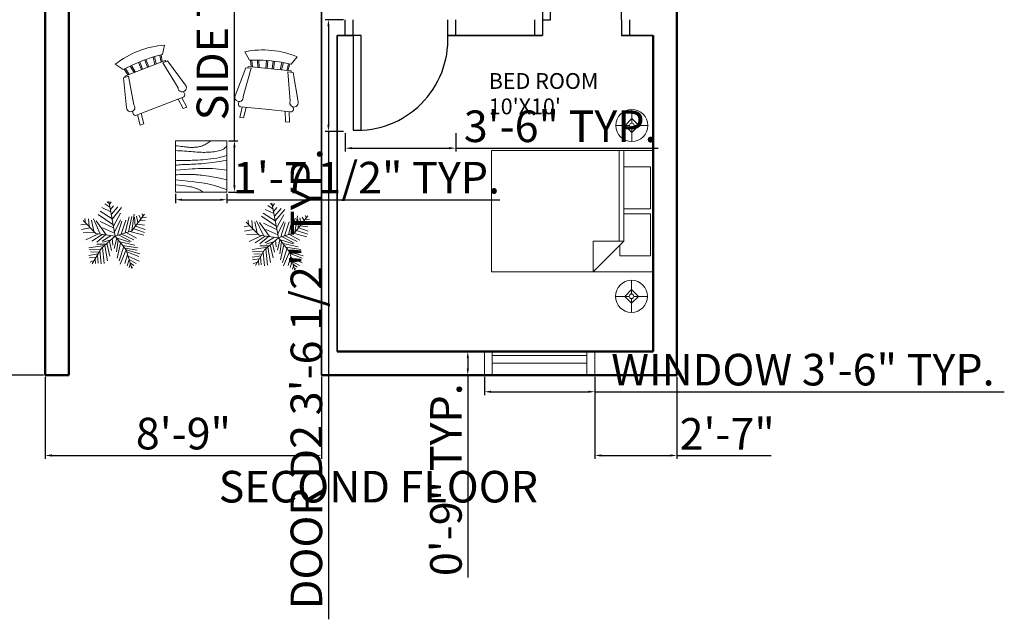
# Model space of a CAD drawing. Units: inches. Extents: x 2296 to 3335, y 495 to 1294.
# Tile 5 of 7: x 2952 to 3326, y 495 to 723. Entities that reach past the tile are written whole.
import ezdxf

# ---------------------------------------------------------------- set-up
doc = ezdxf.new("R2010")
doc.units = ezdxf.units.IN
for name, color, linetype, lineweight in [('A-ANNO-DIMS', 2, 'Continuous', 18), ('A-ANNO-TEXT', 7, 'Continuous', 35), ('A-AREA-IDEN', 7, 'Continuous', 18), ('DOORS', 1, 'Continuous', 25), ('E-LITE', 2, 'Continuous', 18), ('FURNITURE', 2, 'Continuous', 18), ('INNER WALL', 6, 'Continuous', 35), ('L-PLNT', 3, 'Continuous', 13), ('OUTER WALL', 5, 'Continuous', 50), ('WINDOWS', 3, 'Continuous', 18)]:
    doc.layers.add(name, color=color, linetype=linetype, lineweight=lineweight)
doc.styles.get("Standard").update_dxf_attribs({"font": 'arial.ttf'})
doc.dimstyles.new('ISO-25', dxfattribs={"dimtxt": 12, "dimasz": 2.5, "dimexe": 1.25, "dimexo": 0.625, "dimtad": 1, "dimdec": 1, "dimlunit": 3, "dimtxsty": 'Standard', "dimcen": 2.5, "dimadec": 0, "dimazin": 0, "dimtfac": 1, "dimtdec": 1, "dimtmove": 0, "dimatfit": 3, "dimfxl": 1, "dimarcsym": 0})

# ---------------------------------------------------------------- blocks, each defined once
blk = doc.blocks.new('Chair - Rocking')
for p, q in [((-8, -4.5), (-10, -1.5)), ((8, -4.5), (10, -1.5)), ((-8.23428, -6.99939), (-8.3093, -7.47958)), ((-8.23041, -7), (8.23915, -7)), ((-7.5, -4.5), (-7, -7)), ((-6.5, -7), (-7.02225, -4.43)), ((-4.5, -7), (-4.96674, -4.19951)), ((-4, -7), (-4.40532, -4.16272)), ((-1.5, -4.05012), (-1.5, -7)), ((-1, -7), (-1, -4.05012)), ((1, -7), (1, -4.04655)), ((1.5, -4.05012), (1.5, -7)), ((4, -7), (4.40187, -4.18694)), ((4.5, -7), (4.96761, -4.19437)), ((6.5, -7), (7, -4.4057)), ((7.5, -4.5), (7, -7)), ((8.31071, -7.48854), (8.23449, -7.00073)), ((-9, -7.5), (-12, -18.49999)), ((-7, -7.5), (-9, -7.5)), ((-9, -18.49999), (-7, -7.5)), ((7, -7.5), (9, -7.5)), ((9, -18.49999), (7, -7.5)), ((9, -7.5), (12, -18.49999)), ((-10.36644, -20.64523), (-10.5, -21.49999)), ((10.5, -21.49999), (10.3575, -20.58798)), ((-9, -22.49999), (-9.5, -26.49999)), ((0, -22.49999), (-9.5, -22.49999)), ((-8, -26.49999), (-7.5, -22.49999)), ((0, -22.49999), (9.5, -22.49999)), ((8, -26.49999), (7.5, -22.49999)), ((9, -22.49999), (9.5, -26.49999)), ((-9.5, -26.49999), (-8, -26.49999)), ((9.5, -26.49999), (8, -26.49999))]:
    blk.add_line(p, q)
for centre, radius, start, end in [((0, -34.08333), 34.08333, 72.93847, 107.0615), ((0, -68.25004), 64.25, 93.92211, 97.15267), ((0, -68.25004), 64.25, 82.84733, 93.92211), ((-10.5, -18.99999), 1.58114, 161.5651, 18.43495), ((10.5, -18.99999), 1.58114, 161.5651, 18.43495), ((-9.5, -21.49999), 1, 180, 270), ((9.5, -21.49999), 1, 270, 0)]:
    blk.add_arc(centre, radius, start, end)
blk = doc.blocks.new('Table - Square Woodgrain 42 x 42 in.')
blk.add_line((0, -42), (42, -42))
for points in [[(0, -4), (1.704, -4.2172), (3.2358, -4.4188), (4.615, -4.604), (5.8615, -4.7721), (6.9951, -4.9224), (8.0357, -5.0541), (9.0031, -5.1667), (9.9171, -5.2594), (10.7951, -5.3316), (11.6445, -5.3836), (12.4702, -5.4157), (13.277, -5.4283), (14.0698, -5.4217), (14.8535, -5.3964), (15.6331, -5.3526), (16.4133, -5.2908), (17.1986, -5.2103), (17.9913, -5.1062), (18.793, -4.9727), (19.6056, -4.8038), (20.4307, -4.5937), (21.2701, -4.3365), (22.1256, -4.0262), (22.9989, -3.6571), (23.888, -3.2272), (24.7756, -2.7516), (25.6408, -2.2491), (26.4624, -1.7387), (27.2195, -1.2395), (27.891, -0.7703), (28.456, -0.3501), (28.8934, 0.002)], [(0, -42), (0, 0), (42, 0), (42, -42)], [(0, -8), (1.8203, -8.1001), (3.6741, -8.2149), (5.5411, -8.3408), (7.4011, -8.4741), (9.2339, -8.6112), (11.0193, -8.7484), (12.7371, -8.8821), (14.3671, -9.0086), (15.8954, -9.1246), (17.3337, -9.2278), (18.6997, -9.3159), (20.0116, -9.387), (21.2871, -9.4389), (22.5442, -9.4696), (23.8008, -9.477), (25.0749, -9.459), (26.3791, -9.4137), (27.7049, -9.3403), (29.0383, -9.2382), (30.3655, -9.1068), (31.6728, -8.9455), (32.9461, -8.7535), (34.1717, -8.5304), (35.3358, -8.2756), (36.4268, -7.9863), (37.443, -7.6521), (38.3849, -7.2603), (39.253, -6.7986), (40.048, -6.2542), (40.7705, -5.6147), (41.421, -4.8674), (42, -4)], [(42, -12), (39.1784, -12.8621), (36.4519, -13.5654), (33.8246, -14.1294), (31.3004, -14.5731), (28.8832, -14.9161), (26.577, -15.1775), (24.3858, -15.3768), (22.3136, -15.5332), (20.3622, -15.6632), (18.5254, -15.7718), (16.7947, -15.8612), (15.1618, -15.9338), (13.6183, -15.9916), (12.1558, -16.0369), (10.7659, -16.0718), (9.4403, -16.0987), (8.1703, -16.1191), (6.9461, -16.1325), (5.7577, -16.1377), (4.595, -16.1335), (3.4479, -16.1188), (2.3064, -16.0924), (1.1604, -16.0532), (0, -16)], [(42, -16), (37.6529, -16.7365), (33.8802, -17.329), (30.6179, -17.7961), (27.8015, -18.1561), (25.3668, -18.4275), (23.2497, -18.6288), (21.3859, -18.7785), (19.7111, -18.8949), (18.1693, -18.9939), (16.7375, -19.0795), (15.401, -19.1534), (14.1449, -19.217), (12.9544, -19.2717), (11.8148, -19.3191), (10.7113, -19.3606), (9.6291, -19.3976), (8.5534, -19.4323), (7.47, -19.4689), (6.3643, -19.5122), (5.222, -19.5672), (4.0288, -19.6386), (2.7703, -19.7313), (1.4321, -19.8501), (0, -20)], [(0, -24), (3.9243, -23.6805), (7.4766, -23.4138), (10.6891, -23.1954), (13.5943, -23.0205), (16.2247, -22.8847), (18.6125, -22.7832), (20.7903, -22.7116), (22.7903, -22.6651), (24.6563, -22.642), (26.4764, -22.6507), (28.35, -22.7024), (30.3766, -22.8084), (32.6555, -22.98), (35.2861, -23.2283), (38.3678, -23.5645), (42, -24)], [(42, -32), (37.392, -31.017), (33.4585, -30.2231), (30.1291, -29.5949), (27.3334, -29.109), (25.0009, -28.742), (23.0612, -28.4707), (21.4439, -28.2716), (20.0786, -28.1215), (18.8998, -28.0002), (17.8609, -27.9014), (16.9206, -27.8219), (16.0371, -27.7588), (15.1691, -27.709), (14.2748, -27.6693), (13.3128, -27.6368), (12.2415, -27.6083), (11.0295, -27.5824), (9.6867, -27.5643), (8.233, -27.5608), (6.6884, -27.5787), (5.0728, -27.6248), (3.4062, -27.7058), (1.7086, -27.8286), (0, -28)], [(0, -32), (5.4026, -32.5358), (9.9494, -33.019), (13.7424, -33.4553), (16.8834, -33.8505), (19.4743, -34.2106), (21.6171, -34.5413), (23.4136, -34.8486), (24.9657, -35.1382), (26.3614, -35.4156), (27.6332, -35.6841), (28.7995, -35.9467), (29.8788, -36.2064), (30.8897, -36.4661), (31.8507, -36.7288), (32.7802, -36.9973), (33.6968, -37.2747), (34.6175, -37.5635), (35.5531, -37.8651), (36.5128, -38.1805), (37.506, -38.5108), (38.5421, -38.8568), (39.6302, -39.2197), (40.7797, -39.6004), (42, -40)], [(0, -36), (3.0098, -36.2857), (5.5354, -36.5643), (7.6368, -36.8359), (9.374, -37.1009), (10.807, -37.3597), (11.9957, -37.6126), (13.0002, -37.8599), (13.8804, -38.102), (14.6874, -38.3393), (15.4365, -38.5729), (16.1338, -38.8041), (16.7858, -39.0341), (17.3987, -39.264), (17.9787, -39.4952), (18.5322, -39.7288), (19.0655, -39.9662), (19.5832, -40.2081), (20.0842, -40.4544), (20.5657, -40.7046), (21.0249, -40.9581), (21.459, -41.2144), (21.8653, -41.4731), (22.2409, -41.7335), (22.5831, -41.9951)]]:
    blk.add_lwpolyline(points)
blk = doc.blocks.new('Bed - Queen')
for p, q in [((0, -80.00003), (0, 0)), ((0, 0), (59.99999, 0)), ((59.99999, 0), (59.99999, -80.00003)), ((7.99999, -1.2), (28.79998, -1.2)), ((7.99999, -14.4), (7.99999, -1.2)), ((28.79998, -1.2), (28.79998, -14.4)), ((31.19999, -1.2), (51.99999, -1.2)), ((31.19999, -14.4), (31.19999, -1.2)), ((51.99999, -1.2), (51.99999, -16.4)), ((0, -14.4), (44.8, -14.4)), ((59.99999, -29.6), (44.8, -14.4)), ((44.8, -14.4), (44.8, -29.6)), ((44.8, -16.8), (0, -16.8)), ((51.99999, -16.4), (46.79936, -16.4)), ((44.8, -29.6), (59.99999, -29.6)), ((59.99999, -80.00003), (0, -80.00003))]:
    blk.add_line(p, q)
blk = doc.blocks.new('Lamp - Table')
for p, q in [((0, 7), (0, 1)), ((-1, 0), (-7, 0)), ((0, 3), (-3, 0)), ((-3, 0), (0, -3)), ((3, 0), (0, 3)), ((0, -3), (3, 0)), ((1, 0), (7, 0)), ((0, -1), (0, -7))]:
    blk.add_line(p, q)
for radius in [7, 1]:
    blk.add_circle((0, 0), radius)
blk = doc.blocks.new('*U15')
for p, q in [((-8.737, 47.138), (-17.069, 52.711)), ((-10.186, 53.64), (-13.084, 55.962)), ((0, 0), (-10.5, 57)), ((-9.099, 51.782), (-6.563, 55.962)), ((-7.65, 43.423), (-2.578, 49.46)), ((-3.665, 19.273), (-27.574, 35.527)), ((-5.114, 28.097), (-24.676, 40.636)), ((-7.288, 39.707), (-21.778, 46.673)), ((-5.839, 35.992), (4.667, 48.067)), ((-5.114, 27.632), (10.463, 46.673)), ((-2.941, 16.486), (8.652, 37.85)), ((22.055, 7.198), (27.489, 32.277)), ((27, 9), (48, 36)), ((27.127, 9.056), (31.112, 35.992)), ((35.096, 32.741), (37.27, 22.524)), ((38.719, 34.134), (41.979, 28.561)), ((44.153, 36.456), (45.239, 32.741)), ((-47.498, 19.737), (-55.83, 18.344)), ((-31.5, 4.5), (-52.5, 25.5)), ((-48.585, 21.131), (-49.309, 29.026)), ((-43.513, 28.561), (-42.427, 15.558)), ((-38.442, 26.239), (-34.819, 7.663)), ((-35.544, 28.097), (-24.314, 3.947)), ((-14.533, 2.09), (-30.834, 25.31)), ((-24.314, 23.917), (-2.941, 13.7)), ((-1.129, 6.734), (9.014, 26.704)), ((3.942, 1.625), (11.187, 24.381)), ((10.101, 3.483), (17.708, 26.239)), ((16.259, 5.805), (23.142, 31.348)), ((31.836, 30.883), (32.561, 16.486)), ((33.285, 16.486), (48.862, 10.913)), ((36.183, 19.737), (48.137, 17.88)), ((40.53, 25.775), (48.862, 24.846)), ((43.791, 29.954), (51.036, 30.883)), ((-40.615, 13.7), (-55.105, 10.913)), ((-33.37, 6.269), (-52.207, 5.34)), ((-28.299, 3.483), (-47.86, -5.805)), ((-21.416, 3.018), (-38.079, -8.128)), ((0, 0), (-31.5, 4.5)), ((-15.982, 2.09), (-30.11, -9.521)), ((0, 0), (-22.5, -19.5)), ((-6.563, 1.161), (-21.416, -8.128)), ((-20.691, 13.7), (-1.129, 4.876)), ((0, 0), (27, 9)), ((0, 0), (18, -22.5)), ((6.478, 1.625), (26.04, -8.592)), ((11.187, 3.483), (30.749, -5.805)), ((18.07, 5.805), (35.096, -3.483)), ((24.229, 7.663), (46.688, 1.625)), ((29.662, 12.307), (48.137, 6.269)), ((-17.431, -15.094), (-42.789, -18.809)), ((-15.257, -12.772), (-30.11, -12.772)), ((-6.563, -5.805), (-19.967, -9.985)), ((-17.069, -15.094), (-12.721, -40.172)), ((-13.446, -11.378), (-8.737, -32.741)), ((-9.461, -8.592), (-6.201, -23.453)), ((-4.752, -3.483), (-3.665, -14.629)), ((2.493, -3.019), (-1.491, -20.202)), ((1.769, -2.555), (24.229, -9.521)), ((5.029, -6.27), (2.131, -25.775)), ((9.014, -11.378), (3.58, -35.992)), ((7.565, -9.056), (32.198, -14.629)), ((12.274, -15.094), (36.907, -18.809)), ((-28.299, -29.026), (-42.789, -31.348)), ((-24.314, -21.596), (-42.427, -22.06)), ((-26.849, -26.24), (-40.253, -25.775)), ((-22.5, -19.5), (-37.5, -45)), ((-29.023, -30.884), (-27.936, -43.887)), ((-25.038, -23.918), (-22.865, -45.281)), ((-20.691, -18.345), (-17.793, -44.352)), ((14.085, -16.951), (6.478, -40.172)), ((18.07, -22.524), (8.289, -45.745)), ((20.244, -30.419), (15.897, -44.816)), ((16.259, -19.738), (36.183, -22.989)), ((18, -22.5), (27, -52.5)), ((18.433, -22.524), (40.53, -29.026)), ((19.157, -25.311), (38.719, -33.206)), ((-30.834, -34.135), (-42.427, -35.528)), ((-34.457, -39.708), (-40.978, -42.494)), ((-32.646, -36.921), (-31.921, -44.352)), ((22.78, -37.85), (19.519, -48.532)), ((21.331, -32.741), (39.081, -40.636)), ((22.78, -38.314), (34.372, -44.816)), ((24.591, -45.745), (23.142, -50.854)), ((24.591, -43.423), (30.749, -47.603)), ((26.764, -49.925), (28.213, -50.854))]:
    blk.add_line(p, q)
blk = doc.blocks.new('DOOR-SINGLE-30IN')
for p, q in [((-3, 0), (-3, -6)), ((0, 0), (0, -6)), ((30, 0), (30, -6)), ((33, 0), (33, -6))]:
    blk.add_line(p, q)
blk.add_lwpolyline([(0, 0), (3, 0), (3, 30), (0, 30)], close=True)
blk.add_arc((1.5, 1.5), 28.54, 356.9872, 93.0128)
blk = doc.blocks.new('DOOR-SINGLE-36IN')
for p, q in [((0, 39), (-6, 39)), ((0, 36), (-6, 36)), ((0, 0), (-6, 0)), ((0, -3), (-6, -3))]:
    blk.add_line(p, q)
blk.add_lwpolyline([(0, 0), (36, 0), (36, 3), (0, 3)], close=True)
blk.add_arc((1.5, 1.5), 34.53, 357.5104, 92.4896)
blk = doc.blocks.new('WIN-36IN')
for p, q in [((0, 42), (9, 42)), ((0, 39), (9, 39)), ((1.5, 3), (1.5, 39)), ((4.5, 3), (4.5, 39)), ((9, 3), (0, 3)), ((9, 0), (0, 0))]:
    blk.add_line(p, q)
blk = doc.blocks.new('*D35')
at = {"layer": 'A-ANNO-DIMS', "color": 0, "lineweight": -2, "transparency": 16777216}
for p, q in [((3128.54, 587.39), (3128.54, 580.47)), ((3170.54, 587.39), (3170.54, 580.47)), ((3131.04, 581.72), (3168.04, 581.72)), ((3170.54, 581.72), (3326.14, 581.72))]:
    blk.add_line(p, q, dxfattribs=at)
at = {"layer": 'A-ANNO-DIMS', "color": 0, "transparency": 16777216}
for points in [[(3131.04, 582.13), (3131.04, 581.3), (3128.54, 581.72)], [(3168.04, 582.13), (3168.04, 581.3), (3170.54, 581.72)]]:
    blk.add_solid(points, dxfattribs=at)
at = {"layer": 'Defpoints', "color": 0, "transparency": 16777216}
for p in [(3128.54, 588.02), (3170.54, 588.02), (3170.54, 581.72)]:
    blk.add_point(p, dxfattribs=at)
at = {"layer": 'A-ANNO-DIMS', "color": 0, "transparency": 16777216, "insert": (3249.59, 588.56), "char_height": 12, "attachment_point": 5}
blk.add_mtext('WINDOW 3\'-6" TYP.', dxfattribs=at)
blk = doc.blocks.new('*D36')
at = {"layer": 'A-ANNO-DIMS', "color": 0, "lineweight": -2, "transparency": 16777216}
for p, q in [((3127.92, 597.02), (3120.99, 597.02)), ((3122.24, 594.52), (3122.24, 590.52)), ((3127.92, 588.02), (3120.99, 588.02)), ((3122.24, 588.02), (3122.24, 511.12))]:
    blk.add_line(p, q, dxfattribs=at)
at = {"layer": 'A-ANNO-DIMS', "color": 0, "transparency": 16777216}
for points in [[(3121.82, 594.52), (3122.66, 594.52), (3122.24, 597.02)], [(3121.82, 590.52), (3122.66, 590.52), (3122.24, 588.02)]]:
    blk.add_solid(points, dxfattribs=at)
at = {"layer": 'Defpoints', "color": 0, "transparency": 16777216}
for p in [(3128.54, 597.02), (3122.24, 588.02), (3128.54, 588.02)]:
    blk.add_point(p, dxfattribs=at)
at = {"layer": 'A-ANNO-DIMS', "color": 0, "transparency": 16777216, "insert": (3115.49, 548.32), "char_height": 12, "attachment_point": 5, "rotation": 90}
blk.add_mtext('0\'-9" TYP.', dxfattribs=at)
blk = doc.blocks.new('*D39')
at = {"layer": 'A-ANNO-DIMS', "color": 0, "lineweight": -2, "transparency": 16777216}
for p, q in [((3075.02, 723.02), (3068.03, 723.02)), ((3069.28, 720.52), (3069.28, 683.1)), ((3075.02, 680.6), (3068.03, 680.6)), ((3069.28, 680.6), (3069.28, 495.3))]:
    blk.add_line(p, q, dxfattribs=at)
at = {"layer": 'A-ANNO-DIMS', "color": 0, "transparency": 16777216}
for points in [[(3068.87, 720.52), (3069.7, 720.52), (3069.28, 723.02)], [(3068.87, 683.1), (3069.7, 683.1), (3069.28, 680.6)]]:
    blk.add_solid(points, dxfattribs=at)
at = {"layer": 'Defpoints', "color": 0, "transparency": 16777216}
for p in [(3075.65, 723.02), (3069.28, 680.6), (3075.65, 680.6)]:
    blk.add_point(p, dxfattribs=at)
at = {"layer": 'A-ANNO-DIMS', "color": 0, "transparency": 16777216, "insert": (3062.45, 586.7), "char_height": 12, "attachment_point": 5, "rotation": 90}
blk.add_mtext('DOOR D2 3\'-6 1/2" TYP.', dxfattribs=at)
blk = doc.blocks.new('*D40')
at = {"layer": 'A-ANNO-DIMS', "color": 0, "lineweight": -2, "transparency": 16777216}
for p, q in [((3075.65, 679.97), (3075.65, 672.98)), ((3117.65, 679.97), (3117.65, 672.98)), ((3078.15, 674.23), (3115.15, 674.23)), ((3117.65, 674.23), (3194.53, 674.23))]:
    blk.add_line(p, q, dxfattribs=at)
at = {"layer": 'A-ANNO-DIMS', "color": 0, "transparency": 16777216}
for points in [[(3078.15, 674.65), (3078.15, 673.82), (3075.65, 674.23)], [(3115.15, 674.65), (3115.15, 673.82), (3117.65, 674.23)]]:
    blk.add_solid(points, dxfattribs=at)
at = {"layer": 'Defpoints', "color": 0, "transparency": 16777216}
for p in [(3075.65, 680.6), (3117.65, 680.6), (3117.65, 674.23)]:
    blk.add_point(p, dxfattribs=at)
at = {"layer": 'A-ANNO-DIMS', "color": 0, "transparency": 16777216, "insert": (3157.34, 680.99), "char_height": 12, "attachment_point": 5}
blk.add_mtext('3\'-6" TYP.', dxfattribs=at)
blk = doc.blocks.new('*D49')
at = {"layer": 'A-ANNO-DIMS', "color": 0, "lineweight": -2, "transparency": 16777216}
for p, q in [((3033.55, 677.03), (3033.55, 883.38)), ((3031.26, 677.03), (3034.8, 677.03)), ((3033.55, 660.07), (3033.55, 674.53)), ((3031.26, 657.57), (3034.8, 657.57))]:
    blk.add_line(p, q, dxfattribs=at)
at = {"layer": 'A-ANNO-DIMS', "color": 0, "transparency": 16777216}
for points in [[(3033.13, 674.53), (3033.97, 674.53), (3033.55, 677.03)], [(3033.13, 660.07), (3033.97, 660.07), (3033.55, 657.57)]]:
    blk.add_solid(points, dxfattribs=at)
at = {"layer": 'Defpoints', "color": 0, "transparency": 16777216}
for p in [(3030.63, 677.03), (3033.55, 677.03), (3030.63, 657.57)]:
    blk.add_point(p, dxfattribs=at)
at = {"layer": 'A-ANNO-DIMS', "color": 0, "transparency": 16777216, "insert": (3026.72, 781.45), "char_height": 12, "attachment_point": 5, "rotation": 90}
blk.add_mtext('SIDE TABLE 1\'-7 1/2" TYP.', dxfattribs=at)
blk = doc.blocks.new('*D50')
at = {"layer": 'A-ANNO-DIMS', "color": 0, "lineweight": -2, "transparency": 16777216}
for p, q in [((3011.17, 656.94), (3011.17, 653.4)), ((3030.63, 656.94), (3030.63, 653.4)), ((3013.67, 654.65), (3028.13, 654.65)), ((3030.63, 654.65), (3134.36, 654.65))]:
    blk.add_line(p, q, dxfattribs=at)
at = {"layer": 'A-ANNO-DIMS', "color": 0, "transparency": 16777216}
for points in [[(3013.67, 655.07), (3013.67, 654.23), (3011.17, 654.65)], [(3028.13, 655.07), (3028.13, 654.23), (3030.63, 654.65)]]:
    blk.add_solid(points, dxfattribs=at)
at = {"layer": 'Defpoints', "color": 0, "transparency": 16777216}
for p in [(3011.17, 657.57), (3030.63, 657.57), (3030.63, 654.65)]:
    blk.add_point(p, dxfattribs=at)
at = {"layer": 'A-ANNO-DIMS', "color": 0, "transparency": 16777216, "insert": (3083.74, 661.48), "char_height": 12, "attachment_point": 5}
blk.add_mtext('1\'-7 1/2" TYP.', dxfattribs=at)
blk = doc.blocks.new('*D54')
at = {"layer": 'A-ANNO-DIMS', "color": 0, "lineweight": -2, "transparency": 16777216}
for p, q in [((2961.02, 1068.02), (2929.9, 1068.02)), ((2931.15, 590.52), (2931.15, 1065.52)), ((2961.02, 588.02), (2929.9, 588.02))]:
    blk.add_line(p, q, dxfattribs=at)
at = {"layer": 'A-ANNO-DIMS', "color": 0, "transparency": 16777216}
for points in [[(2930.73, 1065.52), (2931.56, 1065.52), (2931.15, 1068.02)], [(2930.73, 590.52), (2931.56, 590.52), (2931.15, 588.02)]]:
    blk.add_solid(points, dxfattribs=at)
at = {"layer": 'Defpoints', "color": 0, "transparency": 16777216}
for p in [(2931.15, 1068.02), (2961.65, 1068.02), (2961.65, 588.02)]:
    blk.add_point(p, dxfattribs=at)
at = {"layer": 'A-ANNO-DIMS', "color": 0, "transparency": 16777216, "insert": (2924.39, 828.02), "char_height": 12, "attachment_point": 5, "rotation": 90}
blk.add_mtext('40\'-0"', dxfattribs=at)
blk = doc.blocks.new('*D77')
at = {"layer": 'A-ANNO-DIMS', "color": 0, "lineweight": -2, "transparency": 16777216}
for p, q in [((3170.54, 587.39), (3170.54, 556.27)), ((3201.65, 587.39), (3201.65, 556.27)), ((3173.04, 557.52), (3199.15, 557.52)), ((3201.65, 557.52), (3237.5, 557.52))]:
    blk.add_line(p, q, dxfattribs=at)
at = {"layer": 'A-ANNO-DIMS', "color": 0, "transparency": 16777216}
for points in [[(3173.04, 557.93), (3173.04, 557.1), (3170.54, 557.52)], [(3199.15, 557.93), (3199.15, 557.1), (3201.65, 557.52)]]:
    blk.add_solid(points, dxfattribs=at)
at = {"layer": 'Defpoints', "color": 0, "transparency": 16777216}
for p in [(3170.54, 588.02), (3201.65, 588.02), (3201.65, 557.52)]:
    blk.add_point(p, dxfattribs=at)
at = {"layer": 'A-ANNO-DIMS', "color": 0, "transparency": 16777216, "insert": (3220.82, 564.17), "char_height": 12, "attachment_point": 5}
blk.add_mtext('2\'-7"', dxfattribs=at)
blk = doc.blocks.new('*D78')
at = {"layer": 'A-ANNO-DIMS', "color": 0, "lineweight": -2, "transparency": 16777216}
for p, q in [((2961.65, 587.39), (2961.65, 556.27)), ((3066.65, 587.39), (3066.65, 556.27)), ((2964.15, 557.52), (3064.15, 557.52))]:
    blk.add_line(p, q, dxfattribs=at)
at = {"layer": 'A-ANNO-DIMS', "color": 0, "transparency": 16777216}
for points in [[(2964.15, 557.93), (2964.15, 557.1), (2961.65, 557.52)], [(3064.15, 557.93), (3064.15, 557.1), (3066.65, 557.52)]]:
    blk.add_solid(points, dxfattribs=at)
at = {"layer": 'Defpoints', "color": 0, "transparency": 16777216}
for p in [(2961.65, 588.02), (3066.65, 588.02), (3066.65, 557.52)]:
    blk.add_point(p, dxfattribs=at)
at = {"layer": 'A-ANNO-DIMS', "color": 0, "transparency": 16777216, "insert": (3014.15, 564.27), "char_height": 12, "attachment_point": 5}
blk.add_mtext('8\'-9"', dxfattribs=at)

msp = doc.modelspace()

# ---------------------------------------------------------------- linework, layer by layer
at = {"layer": 'INNER WALL'}
for p, q in [((3066.65, 588.02), (3066.65, 777.02)), ((3072.65, 717.02), (3078.65, 717.02)), ((3072.65, 597.02), (3072.65, 717.02)), ((3114.65, 717.02), (3150.65, 717.02)), ((3180.65, 717.02), (3192.65, 717.02))]:
    msp.add_line(p, q, dxfattribs=at)
at = {"layer": 'OUTER WALL'}
for p, q in [((2970.65, 861.02), (2970.65, 588.02)), ((3192.65, 597.02), (3192.65, 717.02)), ((3072.65, 597.02), (3192.65, 597.02))]:
    msp.add_line(p, q, dxfattribs=at)
msp.add_lwpolyline([(3066.65, 588.02), (3201.65, 588.02), (3201.65, 1068.02), (2961.65, 1068.02), (2961.65, 588.02), (2970.65, 588.02)], dxfattribs=at)

# ---------------------------------------------------------------- block references
at = {"layer": 'DOORS'}
msp.add_blockref('DOOR-SINGLE-30IN', (3150.65, 723.02), dxfattribs=at)
at = {"layer": 'DOORS', "rotation": 269.9999999999998}
msp.add_blockref('DOOR-SINGLE-36IN', (3078.65, 717.02), dxfattribs=at)
at = {"layer": 'E-LITE', "xscale": 0.8700180084150424, "yscale": 0.8700180084150424, "zscale": 0.8700180084150424}
for p in [(3184.6, 682.84), (3184.47, 617.95)]:
    msp.add_blockref('Lamp - Table', p, dxfattribs=at)
at = {"layer": 'FURNITURE'}
for p, rotation in [((2997.07, 711.13), 21.07995296200778), ((3047.62, 711.37), 354.3621064589386)]:
    msp.add_blockref('Chair - Rocking', p, dxfattribs=dict(at, rotation=rotation))
at = {"layer": 'FURNITURE', "xscale": 0.4632804466850307, "yscale": 0.4632804466850307, "zscale": 0.4632804466850307}
msp.add_blockref('Table - Square Woodgrain 42 x 42 in.', (3011.17, 677.03), dxfattribs=at)
at = {"layer": 'FURNITURE', "xscale": 0.7674836837443932, "yscale": 0.7674836837443932, "zscale": 0.7674836837443932, "rotation": 270}
msp.add_blockref('Bed - Queen', (3192.65, 673.29), dxfattribs=at)
at = {"layer": 'L-PLNT', "xscale": 0.232668267563004, "yscale": 0.232668267563004, "zscale": 0.232668267563004}
for p in [(2988.21, 640.8), (3050.25, 640.14)]:
    msp.add_blockref('*U15', p, dxfattribs=at)
at = {"layer": 'WINDOWS', "rotation": 269.9999999999988}
msp.add_blockref('WIN-36IN', (3128.54, 597.02), dxfattribs=at)

# ---------------------------------------------------------------- texts
at = {"layer": 'A-ANNO-TEXT'}
msp.add_text('SECOND FLOOR', height=12, dxfattribs=at).set_placement((3027.56, 539.66))
at = {"layer": 'A-AREA-IDEN'}
for s, p in [('BED ROOM', (3130.2, 696.74)), ("10'X10'", (3130.2, 687.1))]:
    msp.add_text(s, height=6, dxfattribs=at).set_placement(p)

# ---------------------------------------------------------------- dimensions: what is measured, and where the dimension line sits
at = {"layer": 'A-ANNO-DIMS'}
dim = msp.add_linear_dim(base=(2931.15, 1068.02), p1=(2961.65, 588.02), p2=(2961.65, 1068.02), angle=90, dimstyle='ISO-25', override={"dimdec": 1, "dimlfac": 1, "dimrnd": 0, "dimzin": 1, "dimdsep": 46, "dimlunit": 4, "dimfrac": 2}, dxfattribs=at)
dim.commit()
dim.dimension.update_dxf_attribs({"geometry": '*D54', "text_midpoint": (2924.39, 828.02)})
for base, p1, p2, angle, text, picture, middle in [((3033.55, 677.03), (3030.63, 657.57), (3030.63, 677.03), 90, 'SIDE TABLE <> TYP.', '*D49', (3026.72, 781.45)), ((3069.28, 680.6), (3075.65, 723.02), (3075.65, 680.6), 270, 'DOOR D2 <> TYP.', '*D39', (3062.45, 586.7)), ((3122.24, 588.02), (3128.54, 597.02), (3128.54, 588.02), 270, '<> TYP.', '*D36', (3115.49, 548.32))]:
    dim = msp.add_linear_dim(base=base, p1=p1, p2=p2, angle=angle, text=text, dimstyle='ISO-25', override={"dimdec": 1, "dimlfac": 1, "dimrnd": 0, "dimzin": 1, "dimdsep": 46, "dimlunit": 4, "dimfrac": 2}, dxfattribs=at)
    dim.commit()
    dim.dimension.update_dxf_attribs({"geometry": picture, "text_midpoint": middle})
for base, p1, p2, text, picture, middle in [((3117.65, 674.23), (3075.65, 680.6), (3117.65, 680.6), '<> TYP.', '*D40', (3157.34, 680.99)), ((3030.63, 654.65), (3011.17, 657.57), (3030.63, 657.57), '<> TYP.', '*D50', (3083.74, 661.48)), ((3170.54, 581.72), (3128.54, 588.02), (3170.54, 588.02), 'WINDOW <> TYP.', '*D35', (3249.59, 588.56))]:
    dim = msp.add_linear_dim(base=base, p1=p1, p2=p2, text=text, dimstyle='ISO-25', override={"dimdec": 1, "dimlfac": 1, "dimrnd": 0, "dimzin": 1, "dimdsep": 46, "dimlunit": 4, "dimfrac": 2}, dxfattribs=at)
    dim.commit()
    dim.dimension.update_dxf_attribs({"geometry": picture, "text_midpoint": middle})
for base, p1, p2, picture, middle in [((3066.65, 557.52), (2961.65, 588.02), (3066.65, 588.02), '*D78', (3014.15, 564.27)), ((3201.65, 557.52), (3170.54, 588.02), (3201.65, 588.02), '*D77', (3220.82, 564.17))]:
    dim = msp.add_linear_dim(base=base, p1=p1, p2=p2, dimstyle='ISO-25', override={"dimdec": 1, "dimlfac": 1, "dimrnd": 0, "dimzin": 1, "dimdsep": 46, "dimlunit": 4, "dimfrac": 2}, dxfattribs=at)
    dim.commit()
    dim.dimension.update_dxf_attribs({"geometry": picture, "text_midpoint": middle})

doc.saveas('drawing.dxf')
